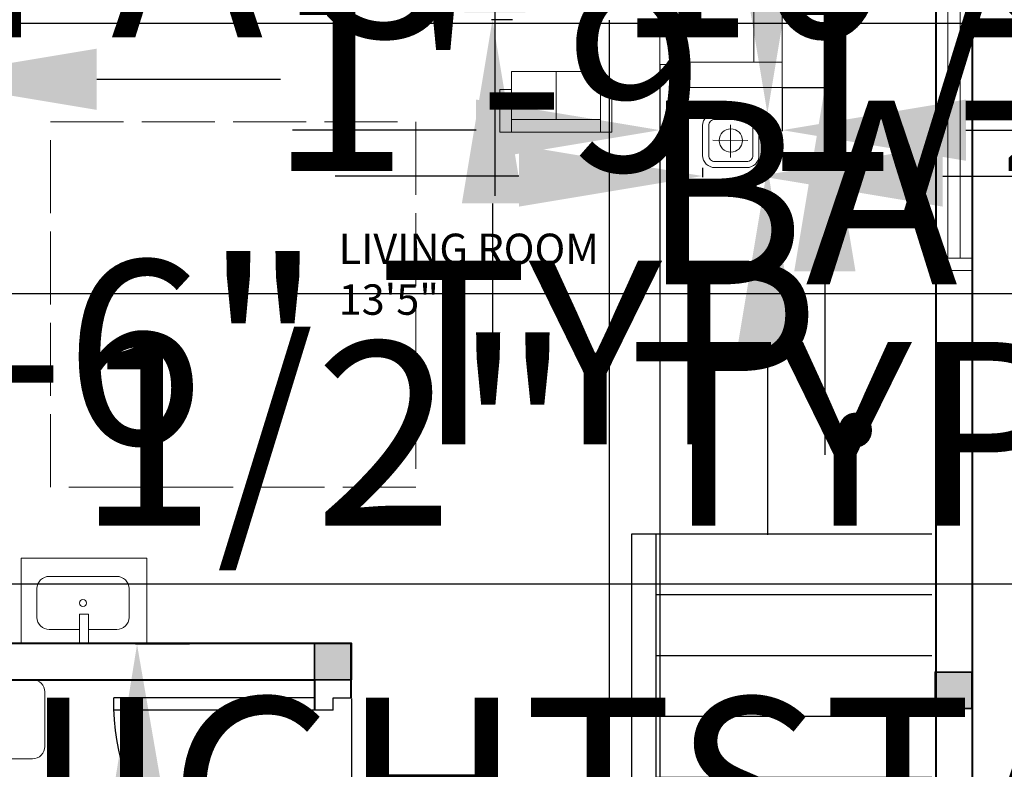
# Model space of a CAD drawing. Units: inches. Extents: x 7323 to 9737, y 2037 to 3322.
# Tile 4 of 19: x 8759 to 8921, y 2297 to 2420. Entities that reach past the tile are written whole.
import ezdxf

# ---------------------------------------------------------------- set-up
doc = ezdxf.new("R2010")
doc.units = ezdxf.units.IN
doc.header["$MEASUREMENT"] = 0
doc.linetypes.add('ACAD_ISO02W100', pattern=[15, 12, -3])
for name, color, linetype, lineweight in [('A-ANNO-DIMS', 2, 'Continuous', 18), ('A-AREA-IDEN', 7, 'Continuous', 18), ('A-COLS', 1, 'Continuous', 35), ('A-DOOR', 4, 'Continuous', 25), ('A-FLOR-CASE', 9, 'Continuous', 20), ('A-FLOR-FIXT', 9, 'Continuous', 18), ('A-FLOR-OVHD', 8, 'ACAD_ISO02W100', 13), ('A-FLOR-STRS', 7, 'Continuous', 25), ('A-FURN', 8, 'Continuous', 18), ('A-GLAZ', 4, 'Continuous', 18), ('A-WALL', 7, 'Continuous', 40)]:
    doc.layers.add(name, color=color, linetype=linetype, lineweight=lineweight)
doc.layers.add('A-COLS-PATT', color=18, linetype='Continuous', lineweight=13, true_color=0x000000)
doc.styles.get("Standard").update_dxf_attribs({"font": 'arial.ttf'})
doc.dimstyles.get("Standard").update_dxf_attribs({"dimtxt": 30.18, "dimasz": 30.18, "dimexe": 0.18, "dimexo": 0.0625, "dimgap": 0.09, "dimtad": 0, "dimtih": 1, "dimtoh": 1, "dimdec": 0, "dimzin": 0, "dimdsep": 46, "dimlunit": 3, "dimtxsty": 'Standard', "dimcen": 0.09, "dimadec": 0, "dimazin": 0, "dimtfac": 1, "dimtdec": 0, "dimtofl": 0, "dimtmove": 0, "dimatfit": 3, "dimfxl": 1, "dimtolj": 1, "dimtzin": 0, "dimarcsym": 0})

# ---------------------------------------------------------------- blocks, each defined once
blk = doc.blocks.new('WIN-48')
for p, q in [((0, 0), (0, 6)), ((2, 0), (2, 6)), ((50, 0), (50, 6)), ((52, 0), (52, 6)), ((2, 4), (50, 4)), ((2, 2), (50, 2))]:
    blk.add_line(p, q)
blk = doc.blocks.new('STAIR-RETURN-FLIGHT')
for p, q in [((45.32, 110), (94.63, 110)), ((45.32, 0), (45.32, 110)), ((49.32, 0), (49.32, 110)), ((49.32, 100), (94.63, 100)), ((49.32, 90), (94.63, 90)), ((49.32, 80), (94.63, 80)), ((49.32, 70), (94.63, 70)), ((49.32, 60), (94.63, 60)), ((49.32, 50), (94.63, 50)), ((0, 40), (45.32, 40)), ((49.32, 40), (94.63, 40)), ((0, 30), (45.32, 30)), ((49.32, 30), (94.63, 30)), ((0, 20), (45.32, 20)), ((49.32, 20), (94.63, 20)), ((0, 10), (45.32, 10)), ((49.32, 10), (94.63, 10)), ((0, 0), (94.63, 0))]:
    blk.add_line(p, q)
blk = doc.blocks.new('DOOR-36')
for p, q in [((33.01, 39), (39.01, 39)), ((36.01, 5), (0.01, 5)), ((36.01, 5), (36.01, 3)), ((33.01, 3), (0.01, 3)), ((36.01, 3), (39.01, 3)), ((33.01, 0), (39.01, 0))]:
    blk.add_line(p, q)
blk.add_arc((35.01, 4), 35.01, 88.3634, 181.6366)
blk = doc.blocks.new('SOFA-THREE-SEAT')
for p, q in [((15.45, 29), (0, 29)), ((15.45, 29), (0, 29)), ((15.45, 15.91), (0, 15.91)), ((15.45, 15.91), (0, 15.91))]:
    blk.add_line(p, q)
for points in [[(20.12, 42.5), (20.12, 42.5), (3.63, 42.5), (3.63, 42.5), (3.63, 46.66), (3.63, 46.66), (20.12, 46.66), (20.12, 46.66)], [(20.12, 42.5), (20.12, 42.5), (3.63, 42.5), (3.63, 42.5), (3.63, 46.66), (3.63, 46.66), (20.12, 46.66), (20.12, 46.66)], [(15.45, 42.5), (15.45, 42.5), (20.12, 42.5), (20.12, 42.5), (20.12, 4.16), (20.12, 4.16), (15.45, 4.16), (15.45, 4.16)], [(15.45, 42.5), (15.45, 42.5), (20.12, 42.5), (20.12, 42.5), (20.12, 4.16), (20.12, 4.16), (15.45, 4.16), (15.45, 4.16)], [(20.12, 0), (20.12, 0), (3.63, 0), (3.63, 0), (3.63, 4.16), (3.63, 4.16), (20.12, 4.16), (20.12, 4.16)], [(20.12, 0), (20.12, 0), (3.63, 0), (3.63, 0), (3.63, 4.16), (3.63, 4.16), (20.12, 4.16), (20.12, 4.16)]]:
    blk.add_lwpolyline(points, close=True)
blk.add_lwpolyline([(15.45, 4.16), (15.45, 42.5), (15.45, 42.5), (0, 42.5), (0, 42.5), (0, 3.77), (0, 3.77), (3.63, 3.77)])
blk.add_lwpolyline([(15.45, 4.16), (15.45, 42.5), (15.45, 42.5), (0, 42.5), (0, 42.5), (0, 3.77), (0, 3.77), (3.63, 3.77)])
blk = doc.blocks.new('ARMCHAIR')
blk.add_line((9.19, 7.87), (9.19, 0))
for points in [[(0, 9.98), (0, 9.98), (1.9, 9.98), (1.9, 9.98), (1.9, 2.97), (1.9, 2.97), (0, 2.97), (0, 2.97)], [(16.51, 7.87), (16.51, 7.87), (1.9, 7.87), (1.9, 7.87), (1.9, 9.98), (1.9, 9.98), (16.51, 9.98), (16.51, 9.98)], [(16.51, 9.95), (16.51, 9.95), (18.41, 9.95), (18.41, 9.95), (18.41, 2.94), (18.41, 2.94), (16.51, 2.94), (16.51, 2.94)], [(16.51, 7.87), (16.51, 7.87), (1.88, 7.87), (1.88, 7.87), (1.88, 0), (1.88, 0), (16.51, 0), (16.51, 0)]]:
    blk.add_lwpolyline(points, close=True)
blk = doc.blocks.new('LOUNGE-SIDE-TABLE')
for p, q in [((4.58, 7.04), (4.58, 1.66)), ((7.42, 4.45), (1.67, 4.53))]:
    blk.add_line(p, q)
for points in [[(9.25, 6.91, 0.414214), (7.25, 8.91), (2, 8.91, 0.414214), (0, 6.91), (0, 2, 0.414214), (2, 0), (7.25, 0, 0.414214), (9.25, 2)], [(8.25, 6.91, 0.414214), (7.25, 7.91), (2, 7.91, 0.414214), (1, 6.91), (1, 2, 0.414214), (2, 1), (7.25, 1, 0.414214), (8.25, 2)]]:
    blk.add_lwpolyline(points, format="xyb", close=True)
blk.add_circle((4.63, 4.45), 1.91)
blk = doc.blocks.new('COL-PLAN-6IN')
blk.add_lwpolyline([(0, 6), (0, 6), (6.06, 6), (6.06, 6), (6.06, 0), (6.06, 0), (0, 0), (0, 0)], close=True)
blk = doc.blocks.new('*D41')
at = {"layer": 'A-ANNO-DIMS', "color": 0, "lineweight": -2, "transparency": 16777216}
for p, q in [((8661.59, 2428.04), (8661.59, 2458.22)), ((8661.59, 2458.22), (8691.77, 2458.22)), ((8657.46, 2397.86), (8661.77, 2397.86)), ((8657.46, 2369.86), (8661.77, 2369.86)), ((8661.59, 2339.68), (8661.59, 2309.5))]:
    blk.add_line(p, q, dxfattribs=at)
at = {"layer": 'A-ANNO-DIMS', "color": 0, "transparency": 16777216}
for points in [[(8656.56, 2428.04), (8666.62, 2428.04), (8661.59, 2397.86)], [(8656.56, 2339.68), (8666.62, 2339.68), (8661.59, 2369.86)]]:
    blk.add_solid(points, dxfattribs=at)
at = {"layer": 'Defpoints', "color": 0, "transparency": 16777216}
for p in [(8657.39, 2397.86), (8661.59, 2397.86), (8657.39, 2369.86)]:
    blk.add_point(p, dxfattribs=at)
at = {"layer": 'A-ANNO-DIMS', "color": 0, "transparency": 16777216, "insert": (8945.06, 2458.22), "char_height": 30.18, "attachment_point": 5}
blk.add_mtext('\\A1;VENT WINDOW 2\'-4" TYP.', dxfattribs=at)
blk = doc.blocks.new('*D42')
at = {"layer": 'A-ANNO-DIMS', "color": 0, "lineweight": -2, "transparency": 16777216}
for p, q in [((8651.39, 2369.8), (8651.39, 2365.48)), ((8657.39, 2369.8), (8657.39, 2365.48)), ((8621.21, 2365.66), (8591.03, 2365.66)), ((8687.57, 2365.66), (8717.75, 2365.66))]:
    blk.add_line(p, q, dxfattribs=at)
at = {"layer": 'A-ANNO-DIMS', "color": 0, "transparency": 16777216}
for points in [[(8621.21, 2370.69), (8621.21, 2360.63), (8651.39, 2365.66)], [(8687.57, 2370.69), (8687.57, 2360.63), (8657.39, 2365.66)]]:
    blk.add_solid(points, dxfattribs=at)
at = {"layer": 'Defpoints', "color": 0, "transparency": 16777216}
for p in [(8651.39, 2369.86), (8657.39, 2369.86), (8657.39, 2365.66)]:
    blk.add_point(p, dxfattribs=at)
at = {"layer": 'A-ANNO-DIMS', "color": 0, "transparency": 16777216, "insert": (8809.82, 2365.66), "char_height": 30.18, "attachment_point": 5}
blk.add_mtext('\\A1;0\'-6" TYP.', dxfattribs=at)
blk = doc.blocks.new('*D43')
at = {"layer": 'A-ANNO-DIMS', "color": 0, "lineweight": -2, "transparency": 16777216}
for p, q in [((9108.94, 2438.75), (9108.94, 2468.93)), ((9104.01, 2408.57), (9109.12, 2408.57)), ((9104.01, 2375.3), (9109.12, 2375.3)), ((9108.94, 2345.12), (9108.94, 2314.94))]:
    blk.add_line(p, q, dxfattribs=at)
at = {"layer": 'A-ANNO-DIMS', "color": 0, "transparency": 16777216}
for points in [[(9103.91, 2438.75), (9113.97, 2438.75), (9108.94, 2408.57)], [(9103.91, 2345.12), (9113.97, 2345.12), (9108.94, 2375.3)]]:
    blk.add_solid(points, dxfattribs=at)
at = {"layer": 'Defpoints', "color": 0, "transparency": 16777216}
for p in [(9103.95, 2408.57), (9108.94, 2408.57), (9103.95, 2375.3)]:
    blk.add_point(p, dxfattribs=at)
at = {"layer": 'A-ANNO-DIMS', "color": 0, "transparency": 16777216, "insert": (9108.94, 2391.93), "char_height": 30.18, "attachment_point": 5}
blk.add_mtext('\\A1;BATH DOOR 2\'-9 1/2" TYP.', dxfattribs=at)
blk = doc.blocks.new('*D47')
at = {"layer": 'A-ANNO-DIMS', "color": 0, "lineweight": -2, "transparency": 16777216}
for p, q in [((8809.55, 2464.49), (8779.37, 2464.49)), ((8839.73, 2461.79), (8839.73, 2464.67)), ((8858.14, 2461.79), (8858.14, 2464.67)), ((8888.32, 2464.49), (8918.5, 2464.49))]:
    blk.add_line(p, q, dxfattribs=at)
at = {"layer": 'A-ANNO-DIMS', "color": 0, "transparency": 16777216}
for points in [[(8809.55, 2469.52), (8809.55, 2459.46), (8839.73, 2464.49)], [(8888.32, 2469.52), (8888.32, 2459.46), (8858.14, 2464.49)]]:
    blk.add_solid(points, dxfattribs=at)
at = {"layer": 'Defpoints', "color": 0, "transparency": 16777216}
for p in [(8858.14, 2464.49), (8839.73, 2461.73), (8858.14, 2461.73)]:
    blk.add_point(p, dxfattribs=at)
at = {"layer": 'A-ANNO-DIMS', "color": 0, "transparency": 16777216, "insert": (9164.9, 2464.49), "char_height": 30.18, "attachment_point": 5}
blk.add_mtext('\\A1;ARMCHAIR 1\'-6 1/2" TYP.', dxfattribs=at)
blk = doc.blocks.new('*D48')
at = {"layer": 'A-ANNO-DIMS', "color": 0, "lineweight": -2, "transparency": 16777216}
for p, q in [((8836.96, 2491.91), (8836.96, 2522.09)), ((8836.96, 2522.09), (8867.14, 2522.09)), ((8839.66, 2461.73), (8836.78, 2461.73)), ((8839.66, 2451.75), (8836.78, 2451.75)), ((8836.96, 2421.57), (8836.96, 2391.39))]:
    blk.add_line(p, q, dxfattribs=at)
at = {"layer": 'A-ANNO-DIMS', "color": 0, "transparency": 16777216}
for points in [[(8831.93, 2491.91), (8841.99, 2491.91), (8836.96, 2461.73)], [(8831.93, 2421.57), (8841.99, 2421.57), (8836.96, 2451.75)]]:
    blk.add_solid(points, dxfattribs=at)
at = {"layer": 'Defpoints', "color": 0, "transparency": 16777216}
for p in [(8836.96, 2461.73), (8839.73, 2461.73), (8839.73, 2451.75)]:
    blk.add_point(p, dxfattribs=at)
at = {"layer": 'A-ANNO-DIMS', "color": 0, "transparency": 16777216, "insert": (8970.94, 2522.09), "char_height": 30.18, "attachment_point": 5}
blk.add_mtext('\\A1;0\'-10" TYP.', dxfattribs=at)
blk = doc.blocks.new('*D49')
at = {"layer": 'A-ANNO-DIMS', "color": 0, "lineweight": -2, "transparency": 16777216}
for p, q in [((8908.77, 2183.8), (8908.77, 2182.67)), ((8915.5, 2183.8), (8915.5, 2182.67)), ((8878.59, 2182.85), (8848.41, 2182.85)), ((8945.68, 2182.85), (8975.86, 2182.85))]:
    blk.add_line(p, q, dxfattribs=at)
at = {"layer": 'A-ANNO-DIMS', "color": 0, "transparency": 16777216}
for points in [[(8878.59, 2187.88), (8878.59, 2177.82), (8908.77, 2182.85)], [(8945.68, 2187.88), (8945.68, 2177.82), (8915.5, 2182.85)]]:
    blk.add_solid(points, dxfattribs=at)
at = {"layer": 'Defpoints', "color": 0, "transparency": 16777216}
for p in [(8908.77, 2183.86), (8915.5, 2183.86), (8915.5, 2182.85)]:
    blk.add_point(p, dxfattribs=at)
at = {"layer": 'A-ANNO-DIMS', "color": 0, "transparency": 16777216, "insert": (9284.58, 2182.85), "char_height": 30.18, "attachment_point": 5}
blk.add_mtext('\\A1;STAIR END POST 0\'-6 1/2" TYP.', dxfattribs=at)
blk = doc.blocks.new('*D53')
at = {"layer": 'A-ANNO-DIMS', "color": 0, "lineweight": -2, "transparency": 16777216}
for p, q in [((8826.85, 2511.06), (8796.67, 2511.06)), ((8857.03, 2503.93), (8857.03, 2511.24)), ((8905.03, 2503.93), (8905.03, 2511.24)), ((8935.21, 2511.06), (8965.39, 2511.06))]:
    blk.add_line(p, q, dxfattribs=at)
at = {"layer": 'A-ANNO-DIMS', "color": 0, "transparency": 16777216}
for points in [[(8826.85, 2516.09), (8826.85, 2506.03), (8857.03, 2511.06)], [(8935.21, 2516.09), (8935.21, 2506.03), (8905.03, 2511.06)]]:
    blk.add_solid(points, dxfattribs=at)
at = {"layer": 'Defpoints', "color": 0, "transparency": 16777216}
for p in [(8905.03, 2511.06), (8857.03, 2503.86), (8905.03, 2503.86)]:
    blk.add_point(p, dxfattribs=at)
at = {"layer": 'A-ANNO-DIMS', "color": 0, "transparency": 16777216, "insert": (9261.3, 2511.06), "char_height": 30.18, "attachment_point": 5}
blk.add_mtext('\\A1;INTERIOR WINDOW 4\'-0" TYP.', dxfattribs=at)
blk = doc.blocks.new('*D63')
at = {"layer": 'A-ANNO-DIMS', "color": 0, "lineweight": -2, "transparency": 16777216}
for p, q in [((8744.72, 2466.22), (8744.72, 2496.4)), ((8744.72, 2496.4), (8774.9, 2496.4)), ((8741.46, 2436.04), (8744.9, 2436.04)), ((8741.46, 2413.86), (8744.9, 2413.86)), ((8744.72, 2383.68), (8744.72, 2353.5))]:
    blk.add_line(p, q, dxfattribs=at)
at = {"layer": 'A-ANNO-DIMS', "color": 0, "transparency": 16777216}
for points in [[(8739.69, 2466.22), (8749.75, 2466.22), (8744.72, 2436.04)], [(8739.69, 2383.68), (8749.75, 2383.68), (8744.72, 2413.86)]]:
    blk.add_solid(points, dxfattribs=at)
at = {"layer": 'Defpoints', "color": 0, "transparency": 16777216}
for p in [(8741.39, 2436.04), (8744.72, 2436.04), (8741.39, 2413.86)]:
    blk.add_point(p, dxfattribs=at)
at = {"layer": 'A-ANNO-DIMS', "color": 0, "transparency": 16777216, "insert": (9003.76, 2496.4), "char_height": 30.18, "attachment_point": 5}
blk.add_mtext('\\A1;APPLIANCE 1\'-10" TYP.', dxfattribs=at)
blk = doc.blocks.new('*D64')
at = {"layer": 'A-ANNO-DIMS', "color": 0, "lineweight": -2, "transparency": 16777216}
for p, q in [((8719.69, 2413.8), (8719.69, 2410.36)), ((8741.39, 2413.8), (8741.39, 2410.36)), ((8689.51, 2410.54), (8659.33, 2410.54)), ((8771.57, 2410.54), (8801.75, 2410.54))]:
    blk.add_line(p, q, dxfattribs=at)
at = {"layer": 'A-ANNO-DIMS', "color": 0, "transparency": 16777216}
for points in [[(8689.51, 2415.57), (8689.51, 2405.51), (8719.69, 2410.54)], [(8771.57, 2415.57), (8771.57, 2405.51), (8741.39, 2410.54)]]:
    blk.add_solid(points, dxfattribs=at)
at = {"layer": 'Defpoints', "color": 0, "transparency": 16777216}
for p in [(8719.69, 2413.86), (8741.39, 2413.86), (8741.39, 2410.54)]:
    blk.add_point(p, dxfattribs=at)
at = {"layer": 'A-ANNO-DIMS', "color": 0, "transparency": 16777216, "insert": (8927.57, 2410.54), "char_height": 30.18, "attachment_point": 5}
blk.add_mtext('\\A1;1\'-9 1/2" TYP.', dxfattribs=at)
blk = doc.blocks.new('*D69')
at = {"layer": 'A-ANNO-DIMS', "color": 0, "lineweight": -2, "transparency": 16777216}
for p, q in [((8836.58, 2472.89), (8836.58, 2503.07)), ((8836.58, 2503.07), (8866.76, 2503.07)), ((8839.88, 2442.71), (8836.4, 2442.71)), ((8839.88, 2420.33), (8836.4, 2420.33)), ((8836.58, 2390.15), (8836.58, 2359.97))]:
    blk.add_line(p, q, dxfattribs=at)
at = {"layer": 'A-ANNO-DIMS', "color": 0, "transparency": 16777216}
for points in [[(8831.55, 2472.89), (8841.61, 2472.89), (8836.58, 2442.71)], [(8831.55, 2390.15), (8841.61, 2390.15), (8836.58, 2420.33)]]:
    blk.add_solid(points, dxfattribs=at)
at = {"layer": 'Defpoints', "color": 0, "transparency": 16777216}
for p in [(8836.58, 2442.71), (8839.94, 2442.71), (8839.94, 2420.33)]:
    blk.add_point(p, dxfattribs=at)
at = {"layer": 'A-ANNO-DIMS', "color": 0, "transparency": 16777216, "insert": (9169.54, 2503.07), "char_height": 30.18, "attachment_point": 5}
blk.add_mtext('\\A1;COFFEE TABLE 1\'-10 1/2" TYP.', dxfattribs=at)
blk = doc.blocks.new('*D70')
at = {"layer": 'A-ANNO-DIMS', "color": 0, "lineweight": -2, "transparency": 16777216}
for p, q in [((8809.76, 2446.06), (8779.58, 2446.06)), ((8839.94, 2442.77), (8839.94, 2446.24)), ((8855.74, 2442.77), (8855.74, 2446.24)), ((8885.92, 2446.06), (8916.1, 2446.06))]:
    blk.add_line(p, q, dxfattribs=at)
at = {"layer": 'A-ANNO-DIMS', "color": 0, "transparency": 16777216}
for points in [[(8809.76, 2451.09), (8809.76, 2441.03), (8839.94, 2446.06)], [(8885.92, 2451.09), (8885.92, 2441.03), (8855.74, 2446.06)]]:
    blk.add_solid(points, dxfattribs=at)
at = {"layer": 'Defpoints', "color": 0, "transparency": 16777216}
for p in [(8855.74, 2446.06), (8839.94, 2442.71), (8855.74, 2442.71)]:
    blk.add_point(p, dxfattribs=at)
at = {"layer": 'A-ANNO-DIMS', "color": 0, "transparency": 16777216, "insert": (9006.75, 2446.06), "char_height": 30.18, "attachment_point": 5}
blk.add_mtext('\\A1;1\'-4" TYP.', dxfattribs=at)
blk = doc.blocks.new('*D71')
at = {"layer": 'A-ANNO-DIMS', "color": 0, "lineweight": -2, "transparency": 16777216}
for p, q in [((8891.18, 2486.02), (8891.18, 2516.2)), ((8884.24, 2455.84), (8891.36, 2455.84)), ((8884.24, 2409.18), (8891.36, 2409.18)), ((8891.18, 2379), (8891.18, 2348.82))]:
    blk.add_line(p, q, dxfattribs=at)
at = {"layer": 'A-ANNO-DIMS', "color": 0, "transparency": 16777216}
for points in [[(8886.15, 2486.02), (8896.21, 2486.02), (8891.18, 2455.84)], [(8886.15, 2379), (8896.21, 2379), (8891.18, 2409.18)]]:
    blk.add_solid(points, dxfattribs=at)
at = {"layer": 'Defpoints', "color": 0, "transparency": 16777216}
for p in [(8884.18, 2455.84), (8891.18, 2455.84), (8884.18, 2409.18)]:
    blk.add_point(p, dxfattribs=at)
at = {"layer": 'A-ANNO-DIMS', "color": 0, "transparency": 16777216, "insert": (8891.18, 2432.51), "char_height": 30.18, "attachment_point": 5}
blk.add_mtext('\\A1;SOFA 3\'-10 1/2" TYP.', dxfattribs=at)
blk = doc.blocks.new('*D72')
at = {"layer": 'A-ANNO-DIMS', "color": 0, "lineweight": -2, "transparency": 16777216}
for p, q in [((8864.06, 2409.12), (8864.06, 2402)), ((8884.18, 2409.12), (8884.18, 2402)), ((8833.88, 2402.18), (8803.7, 2402.18)), ((8914.36, 2402.18), (8944.54, 2402.18))]:
    blk.add_line(p, q, dxfattribs=at)
at = {"layer": 'A-ANNO-DIMS', "color": 0, "transparency": 16777216}
for points in [[(8833.88, 2407.21), (8833.88, 2397.15), (8864.06, 2402.18)], [(8914.36, 2407.21), (8914.36, 2397.15), (8884.18, 2402.18)]]:
    blk.add_solid(points, dxfattribs=at)
at = {"layer": 'Defpoints', "color": 0, "transparency": 16777216}
for p in [(8864.06, 2409.18), (8884.18, 2409.18), (8884.18, 2402.18)]:
    blk.add_point(p, dxfattribs=at)
at = {"layer": 'A-ANNO-DIMS', "color": 0, "transparency": 16777216, "insert": (9035.19, 2402.18), "char_height": 30.18, "attachment_point": 5}
blk.add_mtext('\\A1;1\'-8" TYP.', dxfattribs=at)
blk = doc.blocks.new('*D75')
at = {"layer": 'A-ANNO-DIMS', "color": 0, "lineweight": -2, "transparency": 16777216}
for p, q in [((8629.63, 2293.84), (8599.45, 2293.84)), ((8659.81, 2292), (8659.81, 2294.02)), ((8672.52, 2292), (8672.52, 2294.02)), ((8702.7, 2293.84), (8732.88, 2293.84))]:
    blk.add_line(p, q, dxfattribs=at)
at = {"layer": 'A-ANNO-DIMS', "color": 0, "transparency": 16777216}
for points in [[(8629.63, 2298.87), (8629.63, 2288.81), (8659.81, 2293.84)], [(8702.7, 2298.87), (8702.7, 2288.81), (8672.52, 2293.84)]]:
    blk.add_solid(points, dxfattribs=at)
at = {"layer": 'Defpoints', "color": 0, "transparency": 16777216}
for p in [(8672.52, 2293.84), (8659.81, 2291.93), (8672.52, 2291.93)]:
    blk.add_point(p, dxfattribs=at)
at = {"layer": 'A-ANNO-DIMS', "color": 0, "transparency": 16777216, "insert": (9002.27, 2293.84), "char_height": 30.18, "attachment_point": 5}
blk.add_mtext('\\A1;NIGHTSTAND 1\'-0 1/2" TYP.', dxfattribs=at)
blk = doc.blocks.new('*D76')
at = {"layer": 'A-ANNO-DIMS', "color": 0, "lineweight": -2, "transparency": 16777216}
for p, q in [((8657.91, 2322.11), (8657.91, 2352.29)), ((8657.91, 2352.29), (8688.09, 2352.29)), ((8659.75, 2291.93), (8657.73, 2291.93)), ((8659.75, 2282.32), (8657.73, 2282.32)), ((8657.91, 2252.14), (8657.91, 2221.96))]:
    blk.add_line(p, q, dxfattribs=at)
at = {"layer": 'A-ANNO-DIMS', "color": 0, "transparency": 16777216}
for points in [[(8652.88, 2322.11), (8662.94, 2322.11), (8657.91, 2291.93)], [(8652.88, 2252.14), (8662.94, 2252.14), (8657.91, 2282.32)]]:
    blk.add_solid(points, dxfattribs=at)
at = {"layer": 'Defpoints', "color": 0, "transparency": 16777216}
for p in [(8657.91, 2291.93), (8659.81, 2291.93), (8659.81, 2282.32)]:
    blk.add_point(p, dxfattribs=at)
at = {"layer": 'A-ANNO-DIMS', "color": 0, "transparency": 16777216, "insert": (8815.32, 2352.29), "char_height": 30.18, "attachment_point": 5}
blk.add_mtext('\\A1;0\'-9 1/2" TYP.', dxfattribs=at)
blk = doc.blocks.new('*D79')
at = {"layer": 'A-ANNO-DIMS', "color": 0, "lineweight": -2, "transparency": 16777216}
for p, q in [((8871.1, 2395.97), (8871.1, 2394.46)), ((8880.36, 2395.97), (8880.36, 2394.46)), ((8840.92, 2394.64), (8810.74, 2394.64)), ((8910.54, 2394.64), (8940.72, 2394.64))]:
    blk.add_line(p, q, dxfattribs=at)
at = {"layer": 'A-ANNO-DIMS', "color": 0, "transparency": 16777216}
for points in [[(8840.92, 2399.67), (8840.92, 2389.61), (8871.1, 2394.64)], [(8910.54, 2399.67), (8910.54, 2389.61), (8880.36, 2394.64)]]:
    blk.add_solid(points, dxfattribs=at)
at = {"layer": 'Defpoints', "color": 0, "transparency": 16777216}
for p in [(8871.1, 2396.03), (8880.36, 2396.03), (8880.36, 2394.64)]:
    blk.add_point(p, dxfattribs=at)
at = {"layer": 'A-ANNO-DIMS', "color": 0, "transparency": 16777216, "insert": (9195.57, 2394.64), "char_height": 30.18, "attachment_point": 5}
blk.add_mtext('\\A1;SIDE TABLE 0\'-9 1/2" TYP.', dxfattribs=at)
blk = doc.blocks.new('*D80')
at = {"layer": 'A-ANNO-DIMS', "color": 0, "lineweight": -2, "transparency": 16777216}
for p, q in [((8881.74, 2435.12), (8881.74, 2465.3)), ((8881.74, 2465.3), (8911.92, 2465.3)), ((8880.42, 2404.94), (8881.92, 2404.94)), ((8880.42, 2396.03), (8881.92, 2396.03)), ((8881.74, 2365.85), (8881.74, 2335.67))]:
    blk.add_line(p, q, dxfattribs=at)
at = {"layer": 'A-ANNO-DIMS', "color": 0, "transparency": 16777216}
for points in [[(8876.71, 2435.12), (8886.77, 2435.12), (8881.74, 2404.94)], [(8876.71, 2365.85), (8886.77, 2365.85), (8881.74, 2396.03)]]:
    blk.add_solid(points, dxfattribs=at)
at = {"layer": 'Defpoints', "color": 0, "transparency": 16777216}
for p in [(8880.36, 2404.94), (8881.74, 2404.94), (8880.36, 2396.03)]:
    blk.add_point(p, dxfattribs=at)
at = {"layer": 'A-ANNO-DIMS', "color": 0, "transparency": 16777216, "insert": (9003.99, 2465.3), "char_height": 30.18, "attachment_point": 5}
blk.add_mtext('\\A1;0\'-9" TYP.', dxfattribs=at)
blk = doc.blocks.new('*D97')
at = {"layer": 'A-ANNO-DIMS', "color": 0, "lineweight": -2, "transparency": 16777216}
for p, q in [((8813.39277, 2308.800309), (8813.39277, 2148.482809)), ((8915.39277, 2183.800309), (8915.39277, 2148.482809)), ((8783.21277, 2148.662809), (8753.03277, 2148.662809)), ((8945.57277, 2148.662809), (8975.75277, 2148.662809))]:
    blk.add_line(p, q, dxfattribs=at)
at = {"layer": 'A-ANNO-DIMS', "color": 0, "transparency": 16777216}
for points in [[(8783.21277, 2153.692809), (8783.21277, 2143.632809), (8813.39277, 2148.662809)], [(8945.57277, 2153.692809), (8945.57277, 2143.632809), (8915.39277, 2148.662809)]]:
    blk.add_solid(points, dxfattribs=at)
at = {"layer": 'Defpoints', "color": 0, "transparency": 16777216}
for p in [(8813.39277, 2308.862809), (8915.39277, 2183.862809), (8915.39277, 2148.662809)]:
    blk.add_point(p, dxfattribs=at)
at = {"layer": 'A-ANNO-DIMS', "color": 0, "transparency": 16777216, "insert": (8864.39277, 2148.662809), "char_height": 30.18, "attachment_point": 5}
blk.add_mtext('\\A1;8\'-6"', dxfattribs=at)
blk = doc.blocks.new('*D98')
at = {"layer": 'A-ANNO-DIMS', "color": 0, "lineweight": -2, "transparency": 16777216}
for p, q in [((8813.33, 2317.86), (8778.01, 2317.67)), ((8778.36, 2287.49), (8778.48, 2265.91)), ((8778.77, 2213.85), (8778.65, 2235.43)), ((8814.07, 2183.86), (8778.75, 2183.67))]:
    blk.add_line(p, q, dxfattribs=at)
at = {"layer": 'A-ANNO-DIMS', "color": 0, "transparency": 16777216}
for points in [[(8783.39, 2287.52), (8773.33, 2287.46), (8778.19, 2317.67)], [(8783.79, 2213.88), (8773.74, 2213.82), (8778.93, 2183.67)]]:
    blk.add_solid(points, dxfattribs=at)
at = {"layer": 'Defpoints', "color": 0, "transparency": 16777216}
for p in [(8813.39, 2317.86), (8778.19, 2317.67), (8814.13, 2183.86)]:
    blk.add_point(p, dxfattribs=at)
at = {"layer": 'A-ANNO-DIMS', "color": 0, "transparency": 16777216, "insert": (8778.56, 2250.67), "char_height": 30.18, "attachment_point": 5}
blk.add_mtext('\\A1;11\'-2"', dxfattribs=at)
blk = doc.blocks.new('*D106')
at = {"layer": 'A-ANNO-DIMS', "color": 0, "lineweight": -2, "transparency": 16777216}
for p, q in [((9008.12, 2519.31), (8587.16, 2519.31)), ((8587.34, 2489.13), (8587.34, 2439.14)), ((8587.34, 2357.76), (8587.34, 2407.75)), ((9008.23, 2327.58), (8587.16, 2327.58))]:
    blk.add_line(p, q, dxfattribs=at)
at = {"layer": 'A-ANNO-DIMS', "color": 0, "transparency": 16777216}
for points in [[(8582.31, 2489.13), (8592.37, 2489.13), (8587.34, 2519.31)], [(8582.31, 2357.76), (8592.37, 2357.76), (8587.34, 2327.58)]]:
    blk.add_solid(points, dxfattribs=at)
at = {"layer": 'Defpoints', "color": 0, "transparency": 16777216}
for p in [(8587.34, 2519.31), (9008.18, 2519.31), (9008.29, 2327.58)]:
    blk.add_point(p, dxfattribs=at)
at = {"layer": 'A-ANNO-DIMS', "color": 0, "transparency": 16777216, "insert": (8587.34, 2423.44), "char_height": 30.18, "attachment_point": 5}
blk.add_mtext('\\A1;15\'-11 1/2"', dxfattribs=at)
blk = doc.blocks.new('*D107')
at = {"layer": 'A-ANNO-DIMS', "color": 0, "lineweight": -2, "transparency": 16777216}
for p, q in [((8855.74, 2420.27), (8855.74, 2148.48)), ((8864.06, 2412.89), (8864.06, 2148.48)), ((8825.56, 2148.66), (8795.38, 2148.66)), ((8894.24, 2148.66), (8924.42, 2148.66))]:
    blk.add_line(p, q, dxfattribs=at)
at = {"layer": 'A-ANNO-DIMS', "color": 0, "transparency": 16777216}
for points in [[(8825.56, 2153.69), (8825.56, 2143.63), (8855.74, 2148.66)], [(8894.24, 2153.69), (8894.24, 2143.63), (8864.06, 2148.66)]]:
    blk.add_solid(points, dxfattribs=at)
at = {"layer": 'Defpoints', "color": 0, "transparency": 16777216}
for p in [(8855.74, 2420.33), (8864.06, 2412.95), (8864.06, 2148.66)]:
    blk.add_point(p, dxfattribs=at)
at = {"layer": 'A-ANNO-DIMS', "color": 0, "transparency": 16777216, "insert": (8999.78, 2148.66), "char_height": 30.18, "attachment_point": 5}
blk.add_mtext('\\A1;0\'-8 1/2"', dxfattribs=at)
blk = doc.blocks.new('*D108')
at = {"layer": 'A-ANNO-DIMS', "color": 0, "lineweight": -2, "transparency": 16777216}
for p, q in [((8587.34, 2481.93), (8587.34, 2512.11)), ((8841.54, 2451.75), (8587.16, 2451.75)), ((8839.88, 2442.71), (8587.16, 2442.71)), ((8587.34, 2412.53), (8587.34, 2382.35)), ((8587.34, 2382.35), (8557.16, 2382.35))]:
    blk.add_line(p, q, dxfattribs=at)
at = {"layer": 'A-ANNO-DIMS', "color": 0, "transparency": 16777216}
for points in [[(8582.31, 2481.93), (8592.37, 2481.93), (8587.34, 2451.75)], [(8582.31, 2412.53), (8592.37, 2412.53), (8587.34, 2442.71)]]:
    blk.add_solid(points, dxfattribs=at)
at = {"layer": 'Defpoints', "color": 0, "transparency": 16777216}
for p in [(8841.6, 2451.75), (8587.34, 2442.71), (8839.94, 2442.71)]:
    blk.add_point(p, dxfattribs=at)
at = {"layer": 'A-ANNO-DIMS', "color": 0, "transparency": 16777216, "insert": (8516.96, 2382.35), "char_height": 30.18, "attachment_point": 5}
blk.add_mtext('\\A1;0\'-9"', dxfattribs=at)
blk = doc.blocks.new('*D110')
at = {"layer": 'A-ANNO-DIMS', "color": 0, "lineweight": -2, "transparency": 16777216}
for p, q in [((8587.34, 2449.91), (8587.34, 2480.09)), ((9018.85, 2419.73), (8587.16, 2419.73)), ((9018.85, 2375.3), (8587.16, 2375.3)), ((8587.34, 2345.12), (8587.34, 2314.94))]:
    blk.add_line(p, q, dxfattribs=at)
at = {"layer": 'A-ANNO-DIMS', "color": 0, "transparency": 16777216}
for points in [[(8582.31, 2449.91), (8592.37, 2449.91), (8587.34, 2419.73)], [(8582.31, 2345.12), (8592.37, 2345.12), (8587.34, 2375.3)]]:
    blk.add_solid(points, dxfattribs=at)
at = {"layer": 'Defpoints', "color": 0, "transparency": 16777216}
for p in [(8587.34, 2419.73), (9018.91, 2419.73), (9018.91, 2375.3)]:
    blk.add_point(p, dxfattribs=at)
at = {"layer": 'A-ANNO-DIMS', "color": 0, "transparency": 16777216, "insert": (8587.34, 2397.51), "char_height": 30.18, "attachment_point": 5}
blk.add_mtext('\\A1;3\'-8 1/2"', dxfattribs=at)
blk = doc.blocks.new('*D127')
at = {"layer": 'A-ANNO-DIMS', "color": 0, "lineweight": -2, "transparency": 16777216}
for p, q in [((9006.57, 2442.49), (9036.75, 2442.49)), ((9036.75, 2442.49), (9058.09, 2421.15)), ((9099.86, 2379.3), (9100.04, 2379.3)), ((9099.95, 2379.21), (9099.95, 2379.39))]:
    blk.add_line(p, q, dxfattribs=at)
at = {"layer": 'A-ANNO-DIMS', "color": 0, "transparency": 16777216}
blk.add_solid([(9061.64, 2424.71), (9054.53, 2417.6), (9079.43, 2399.81)], dxfattribs=at)
at = {"layer": 'Defpoints', "color": 0, "transparency": 16777216}
for p in [(9079.43, 2399.81), (9099.95, 2379.3)]:
    blk.add_point(p, dxfattribs=at)
at = {"layer": 'A-ANNO-DIMS', "color": 0, "transparency": 16777216, "insert": (8951.92, 2442.49), "char_height": 30.18, "attachment_point": 5}
blk.add_mtext('\\A1;R2\'-5"', dxfattribs=at)

msp = doc.modelspace()

# ---------------------------------------------------------------- hatches: boundary and pattern name
at = {"layer": 'A-COLS-PATT'}
h = msp.add_hatch(color=256, dxfattribs=at)
h.dxf.hatch_style = 1
h.paths.add_polyline_path([(8915.39, 2189.86), (8908.77, 2189.86), (8908.77, 2183.86), (8915.39, 2183.86)])
h.paths.add_polyline_path([(8657.61, 2189.86), (8651.55, 2189.86), (8651.55, 2183.86), (8657.61, 2183.86)])
h.paths.add_polyline_path([(8814.13, 2189.86), (8807.39, 2189.86), (8807.39, 2183.86), (8814.13, 2183.86)])
h.paths.add_polyline_path([(8813.39, 2317.86), (8807.36, 2317.86), (8807.36, 2311.86), (8813.39, 2311.86)])
h.paths.add_polyline_path([(8915.34, 2313.13), (8909.39, 2313.13), (8909.39, 2307.13), (8915.34, 2307.13)])
h.paths.add_polyline_path([(8657.62, 2317.86), (8657.39, 2317.86), (8657.39, 2318.08), (8651.55, 2318.08), (8651.55, 2312.08), (8657.62, 2312.08)])
h.paths.add_polyline_path([(8915.39, 2671.84), (8909.37, 2671.84), (8909.37, 2665.86), (8909.39, 2665.86), (8915.39, 2665.84)])
h.paths.add_polyline_path([(8657.59, 2671.81), (8651.52, 2671.81), (8651.52, 2665.81), (8657.39, 2665.81), (8657.39, 2665.86)])
h.paths.add_polyline_path([(8915.28, 2503.94), (8909.39, 2503.94), (8909.39, 2503.86), (8909.22, 2497.94), (8915.28, 2497.94)])
h.paths.add_polyline_path([(8657.53, 2503.86), (8657.39, 2503.86), (8651.46, 2503.96), (8651.46, 2497.96), (8657.53, 2497.96)])
h.paths.add_polyline_path([(9014.24, 2519.3), (9013.95, 2519.3), (9008.18, 2519.31), (9008.18, 2513.31), (9014.24, 2513.31)])
h.paths.add_polyline_path([(9013.95, 2687.3), (9007.95, 2687.3), (9007.95, 2681.3), (9013.95, 2681.3)])
h.paths.add_polyline_path([(9271.95, 2687.3), (9266.01, 2687.3), (9266.01, 2681.35), (9271.95, 2681.35)])
h.paths.add_polyline_path([(9271.95, 2205.3), (9265.32, 2205.3), (9265.32, 2199.3), (9271.95, 2199.3)])
h.paths.add_polyline_path([(9170.68, 2205.3), (9163.95, 2205.3), (9163.95, 2199.3), (9170.68, 2199.3)])
h.paths.add_polyline_path([(9013.95, 2205.3), (9007.95, 2205.3), (9007.95, 2199.3), (9013.95, 2199.3)])
h.paths.add_polyline_path([(9271.95, 2519.51), (9265.95, 2519.51), (9265.95, 2519.3), (9265.93, 2513.51), (9271.95, 2513.51)])
h.paths.add_polyline_path([(9271.95, 2328.64), (9265.95, 2328.64), (9265.95, 2322.64), (9271.95, 2322.64)])
h.paths.add_polyline_path([(9014.35, 2333.3), (9013.95, 2333.3), (9013.95, 2333.58), (9008.29, 2333.58), (9008.29, 2327.58), (9014.35, 2327.58)])

# ---------------------------------------------------------------- linework, layer by layer
at = {"layer": 'A-FLOR-CASE'}
msp.add_lwpolyline([(8676.4, 2300.88, 0.414214), (8678.4, 2298.88), (8761.03, 2298.88, 0.414214), (8763.03, 2300.88), (8763.03, 2309.86, 0.414214), (8761.03, 2311.86), (8678.4, 2311.86, 0.414214), (8676.4, 2309.86)], format="xyb", close=True, dxfattribs=at)
at = {"layer": 'A-FLOR-FIXT'}
for points in [[(8759.18, 2317.86), (8759.18, 2317.86), (8779.8, 2317.86), (8779.8, 2317.86), (8779.8, 2331.83), (8779.8, 2331.83), (8759.18, 2331.83), (8759.18, 2331.83)], [(8770.23, 2317.86), (8770.23, 2317.86), (8768.75, 2317.86), (8768.75, 2317.86), (8768.75, 2322.63), (8768.75, 2322.63), (8770.23, 2322.63), (8770.23, 2322.63)]]:
    msp.add_lwpolyline(points, close=True, dxfattribs=at)
msp.add_lwpolyline([(8768.75, 2320.11), (8763.75, 2320.11, -0.414214), (8761.75, 2322.11), (8761.75, 2326.84, -0.414214), (8763.75, 2328.84), (8774.87, 2328.84, -0.414214), (8776.87, 2326.84), (8776.87, 2322.11, -0.414214), (8774.87, 2320.11), (8770.23, 2320.11)], format="xyb", dxfattribs=at)
msp.add_circle((8769.31, 2324.47), 0.568, dxfattribs=at)
at = {"layer": 'A-FLOR-OVHD'}
for p, q in [((8763.98, 2403.53), (8823.98, 2403.53)), ((8763.98, 2343.53), (8763.98, 2403.53)), ((8823.98, 2403.53), (8823.98, 2343.53)), ((8823.98, 2343.53), (8763.98, 2343.53))]:
    msp.add_line(p, q, dxfattribs=at)
at = {"layer": 'A-WALL'}
for p, q in [((8915.39, 2671.86), (8915.39, 2183.86)), ((8909.39, 2497.86), (8909.39, 2189.86)), ((8747.39, 2317.86), (8813.39, 2317.86)), ((8813.39, 2308.86), (8813.39, 2317.86)), ((8657.39, 2311.86), (8807.39, 2311.86)), ((8807.39, 2306.86), (8807.39, 2311.86))]:
    msp.add_line(p, q, dxfattribs=at)

# ---------------------------------------------------------------- block references
at = {"layer": 'A-COLS'}
for p in [(8807.36, 2311.86), (8909.28, 2307.13)]:
    msp.add_blockref('COL-PLAN-6IN', p, dxfattribs=at)
at = {"layer": 'A-DOOR', "extrusion": (0, 0, -1), "zscale": -1, "rotation": 180}
msp.add_blockref('DOOR-36', (-8774.38, 2311.86), dxfattribs=at)
at = {"layer": 'A-FLOR-STRS'}
msp.add_blockref('STAIR-RETURN-FLIGHT', (8814.13, 2225.86), dxfattribs=at)
at = {"layer": 'A-FURN'}
for name, p in [('SOFA-THREE-SEAT', (8864.06, 2409.18)), ('LOUNGE-SIDE-TABLE', (8871.1, 2396.03))]:
    msp.add_blockref(name, p, dxfattribs=at)
at = {"layer": 'A-FURN', "rotation": 180}
msp.add_blockref('ARMCHAIR', (8856.21, 2411.81), dxfattribs=at)
at = {"layer": 'A-GLAZ', "rotation": 89.99999999999191}
msp.add_blockref('WIN-48', (8915.39, 2379.12), dxfattribs=at)

# ---------------------------------------------------------------- texts
at = {"layer": 'A-AREA-IDEN', "insert": (8811.3, 2385.17), "char_height": 5, "attachment_point": 1}
msp.add_mtext_dynamic_manual_height_columns('LIVING ROOM\\P13\'5"', width=54.2256, gutter_width=1, heights=[0], dxfattribs=at)

# ---------------------------------------------------------------- dimensions: what is measured, and where the dimension line sits
at = {"layer": 'A-ANNO-DIMS'}
for base, p1, p2, text, picture, middle in [((8836.58, 2442.71), (8839.94, 2420.33), (8839.94, 2442.71), 'COFFEE TABLE <> TYP.', '*D69', (9169.54, 2503.07)), ((8836.96, 2461.73), (8839.73, 2451.75), (8839.73, 2461.73), '<> TYP.', '*D48', (8970.94, 2522.09)), ((8744.72, 2436.04), (8741.39, 2413.86), (8741.39, 2436.04), 'APPLIANCE <> TYP.', '*D63', (9003.76, 2496.4)), ((8661.59, 2397.86), (8657.39, 2369.86), (8657.39, 2397.86), 'VENT WINDOW <> TYP.', '*D41', (8945.06, 2458.22)), ((8891.18, 2455.84), (8884.18, 2409.18), (8884.18, 2455.84), 'SOFA <> TYP.', '*D71', (8891.18, 2432.51)), ((9108.94, 2408.57), (9103.95, 2375.3), (9103.95, 2408.57), 'BATH DOOR <> TYP.', '*D43', (9108.94, 2391.93)), ((8881.74, 2404.94), (8880.36, 2396.03), (8880.36, 2404.94), '<> TYP.', '*D80', (9003.99, 2465.3)), ((8657.91, 2291.93), (8659.81, 2282.32), (8659.81, 2291.93), '<> TYP.', '*D76', (8815.32, 2352.29))]:
    dim = msp.add_linear_dim(base=base, p1=p1, p2=p2, angle=90, text=text, dimstyle='Standard', override={"dimdec": 1, "dimlfac": 1, "dimrnd": 0, "dimzin": 1, "dimdsep": 46, "dimlunit": 4, "dimfrac": 2}, dxfattribs=at)
    dim.commit()
    dim.dimension.update_dxf_attribs({"geometry": picture, "text_midpoint": middle})
for base, p1, p2, text, picture, middle in [((8905.03, 2511.06), (8857.03, 2503.86), (8905.03, 2503.86), 'INTERIOR WINDOW <> TYP.', '*D53', (9261.3, 2511.06)), ((8858.14, 2464.49), (8839.73, 2461.73), (8858.14, 2461.73), 'ARMCHAIR <> TYP.', '*D47', (9164.9, 2464.49)), ((8880.36, 2394.64), (8871.1, 2396.03), (8880.36, 2396.03), 'SIDE TABLE <> TYP.', '*D79', (9195.57, 2394.64)), ((8855.74, 2446.06), (8839.94, 2442.71), (8855.74, 2442.71), '<> TYP.', '*D70', (9006.75, 2446.06)), ((8741.39, 2410.54), (8719.69, 2413.86), (8741.39, 2413.86), '<> TYP.', '*D64', (8927.57, 2410.54)), ((8884.18, 2402.18), (8864.06, 2409.18), (8884.18, 2409.18), '<> TYP.', '*D72', (9035.19, 2402.18)), ((8657.39, 2365.66), (8651.39, 2369.86), (8657.39, 2369.86), '<> TYP.', '*D42', (8809.82, 2365.66)), ((8672.52, 2293.84), (8659.81, 2291.93), (8672.52, 2291.93), 'NIGHTSTAND <> TYP.', '*D75', (9002.27, 2293.84)), ((8915.5, 2182.85), (8908.77, 2183.86), (8915.5, 2183.86), 'STAIR END POST <> TYP.', '*D49', (9284.58, 2182.85))]:
    dim = msp.add_linear_dim(base=base, p1=p1, p2=p2, text=text, dimstyle='Standard', override={"dimdec": 1, "dimlfac": 1, "dimrnd": 0, "dimzin": 1, "dimdsep": 46, "dimlunit": 4, "dimfrac": 2}, dxfattribs=at)
    dim.commit()
    dim.dimension.update_dxf_attribs({"geometry": picture, "text_midpoint": middle})
for base, p1, p2, angle, picture, middle in [((8587.34, 2519.31), (9008.29, 2327.58), (9008.18, 2519.31), 90, '*D106', (8587.34, 2423.44)), ((8587.34, 2442.71), (8841.6, 2451.75), (8839.94, 2442.71), 90, '*D108', (8516.96, 2382.35)), ((8587.34, 2419.73), (9018.91, 2375.3), (9018.91, 2419.73), 90, '*D110', (8587.34, 2397.51)), ((8778.19, 2317.67), (8814.13, 2183.86), (8813.39, 2317.86), 90.3155, '*D98', (8778.56, 2250.67))]:
    dim = msp.add_linear_dim(base=base, p1=p1, p2=p2, angle=angle, dimstyle='Standard', override={"dimdec": 1, "dimlfac": 1, "dimrnd": 0, "dimzin": 1, "dimdsep": 46, "dimlunit": 4, "dimfrac": 2}, dxfattribs=at)
    dim.commit()
    dim.dimension.update_dxf_attribs({"geometry": picture, "text_midpoint": middle})
dim = msp.add_radius_dim(center=(9099.95, 2379.3), mpoint=(9079.43, 2399.81), dimstyle='Standard', override={"dimdec": 1, "dimlfac": 1, "dimrnd": 0, "dimzin": 1, "dimdsep": 46, "dimlunit": 4, "dimfrac": 2}, dxfattribs=at)
dim.commit()
dim.dimension.update_dxf_attribs({"geometry": '*D127', "text_midpoint": (8951.92, 2442.49)})
for base, p1, p2, picture, middle in [((8864.06, 2148.66), (8855.74, 2420.33), (8864.06, 2412.95), '*D107', (8999.78, 2148.66)), ((8915.39, 2148.66), (8813.39, 2308.86), (8915.39, 2183.86), '*D97', (8864.39, 2148.66))]:
    dim = msp.add_linear_dim(base=base, p1=p1, p2=p2, dimstyle='Standard', override={"dimdec": 1, "dimlfac": 1, "dimrnd": 0, "dimzin": 1, "dimdsep": 46, "dimlunit": 4, "dimfrac": 2}, dxfattribs=at)
    dim.commit()
    dim.dimension.update_dxf_attribs({"geometry": picture, "text_midpoint": middle})

doc.saveas('drawing.dxf')
